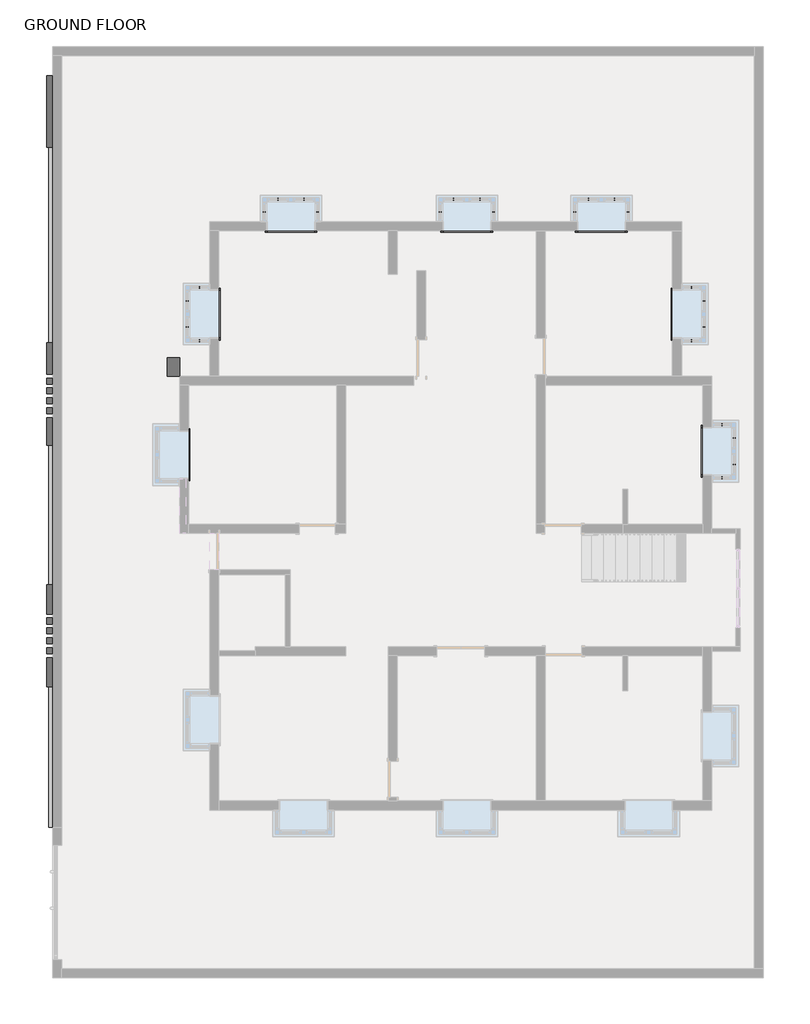
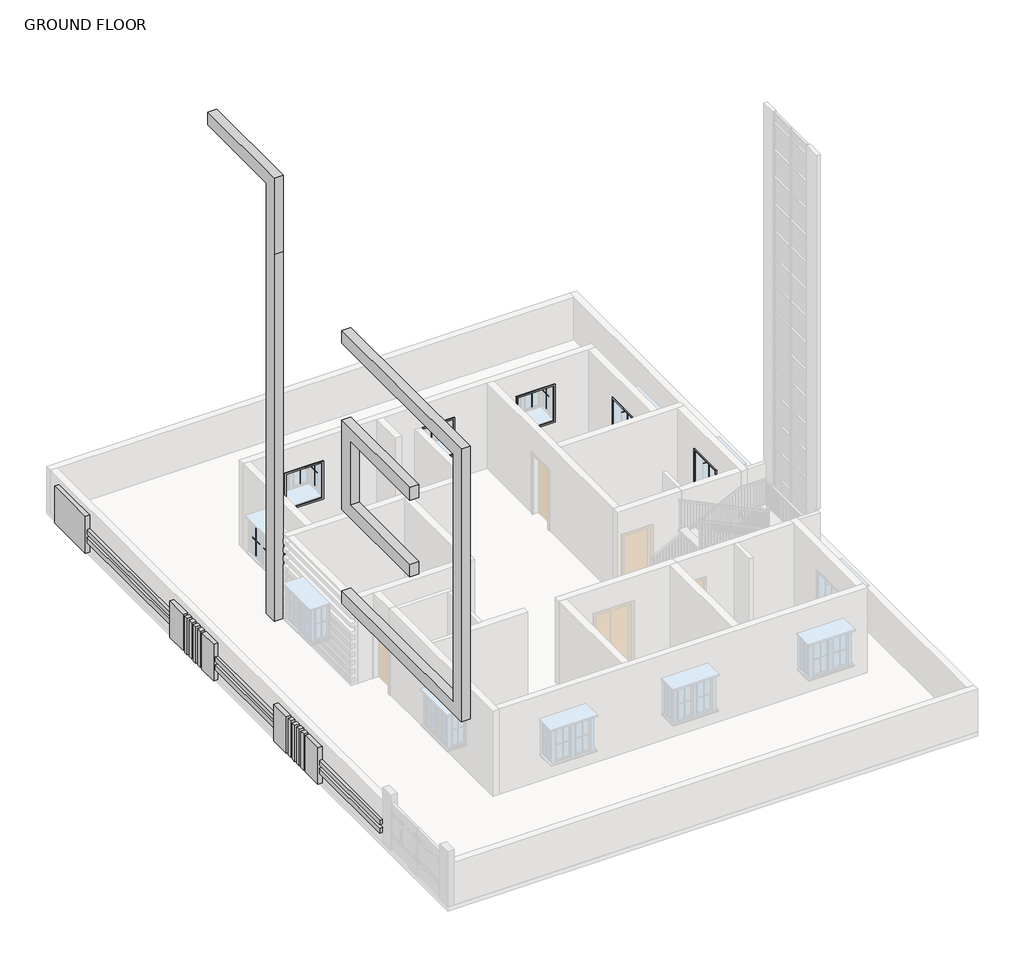
# One storey, part 5 of 5: 32 proxies.
"""IFC4 building model written with IfcOpenShell, lengths in millimetres."""

from ifc_helpers import new_model, si_unit, origin, place, context, project, spatial, transform, mapped, element, save
from components import generic_models_2_generic_models_2_d91b4525, muntin_pattern_2x2_muntin_pattern_2x2_4aee108e, muntin_pattern_2x2_muntin_pattern_2x2_f03ab90d, muntin_pattern_2x2_muntin_pattern_2x2_eb08c668, trim_window_interior_flat_picture_frame_ace0ae79

model = new_model("IFC4")

# Units and contexts
model_context = context("Model", 3, world=origin())
ifc_project = project(units=[si_unit("LENGTHUNIT", "METRE", prefix="MILLI")], contexts=[model_context])

# Site, building, storey
site = spatial("IfcSite", under=ifc_project)
building = spatial("IfcBuilding", under=site)
storey = spatial("IfcBuildingStorey", under=building, Name="GROUND FLOOR", Elevation=0.0)

# Proxies
placement = place(None, origin())
generic_models_2_generic_models_2_shape = generic_models_2_generic_models_2_d91b4525(model_context)
element("IfcBuildingElementProxy", 1, Name="Generic Models 2 : Generic Models 2", ObjectType="Generic Models 2 : Generic Models 2", at=placement, inside=storey, context=model_context, shape_type="MappedRepresentation", body=[
    mapped(generic_models_2_generic_models_2_shape, transform((0.0, 0.0, 0.0), x_axis=(1.0, 0.0, 0.0), y_axis=(0.0, 1.0, 0.0), z_axis=(0.0, 0.0, 1.0))),
])
muntin_pattern_2x2_muntin_pattern_2x2_shape = muntin_pattern_2x2_muntin_pattern_2x2_4aee108e(model_context)
element("IfcBuildingElementProxy", 2, Name="Muntin Pattern_2x2 : Muntin Pattern_2x2", ObjectType="Muntin Pattern_2x2 : Muntin Pattern_2x2", at=placement, inside=storey, context=model_context, shape_type="MappedRepresentation", body=[
    mapped(muntin_pattern_2x2_muntin_pattern_2x2_shape, transform((6209.1834916, 6075.433346, 1035.05), x_axis=(0.0, -1.0, 0.0), y_axis=(1.0, 0.0, 0.0), z_axis=(0.0, 0.0, 1.0))),
])
element("IfcBuildingElementProxy", 3, Name="Muntin Pattern_2x2 : Muntin Pattern_2x2", ObjectType="Muntin Pattern_2x2 : Muntin Pattern_2x2", at=placement, inside=storey, context=model_context, shape_type="MappedRepresentation", body=[
    mapped(muntin_pattern_2x2_muntin_pattern_2x2_shape, transform((-6814.6665084, 5415.033346, 1035.05), x_axis=(0.0, 1.0, 0.0), y_axis=(-1.0, 0.0, 0.0), z_axis=(0.0, 0.0, 1.0))),
])
element("IfcBuildingElementProxy", 4, Name="Muntin Pattern_2x2 : Muntin Pattern_2x2", ObjectType="Muntin Pattern_2x2 : Muntin Pattern_2x2", at=placement, inside=storey, context=model_context, shape_type="MappedRepresentation", body=[
    mapped(muntin_pattern_2x2_muntin_pattern_2x2_shape, transform((-99.5415084, 8637.658346, 1035.05), x_axis=(1.0, 0.0, 0.0), y_axis=(0.0, 1.0, 0.0), z_axis=(0.0, 0.0, 1.0))),
])
element("IfcBuildingElementProxy", 5, Name="Muntin Pattern_2x2 : Muntin Pattern_2x2", ObjectType="Muntin Pattern_2x2 : Muntin Pattern_2x2", at=placement, inside=storey, context=model_context, shape_type="MappedRepresentation", body=[
    mapped(muntin_pattern_2x2_muntin_pattern_2x2_shape, transform((3291.3584916, 8637.658346, 1035.05), x_axis=(1.0, 0.0, 0.0), y_axis=(0.0, 1.0, 0.0), z_axis=(0.0, 0.0, 1.0))),
])
element("IfcBuildingElementProxy", 6, Name="Muntin Pattern_2x2 : Muntin Pattern_2x2", ObjectType="Muntin Pattern_2x2 : Muntin Pattern_2x2", at=placement, inside=storey, context=model_context, shape_type="MappedRepresentation", body=[
    mapped(muntin_pattern_2x2_muntin_pattern_2x2_shape, transform((-4531.8415084, 8637.658346, 1035.05), x_axis=(1.0, 0.0, 0.0), y_axis=(0.0, 1.0, 0.0), z_axis=(0.0, 0.0, 1.0))),
])
element("IfcBuildingElementProxy", 7, Name="Muntin Pattern_2x2 : Muntin Pattern_2x2", ObjectType="Muntin Pattern_2x2 : Muntin Pattern_2x2", at=placement, inside=storey, context=model_context, shape_type="MappedRepresentation", body=[
    mapped(muntin_pattern_2x2_muntin_pattern_2x2_shape, transform((6971.1834916, 2621.033346, 1035.05), x_axis=(0.0, -1.0, 0.0), y_axis=(1.0, 0.0, 0.0), z_axis=(0.0, 0.0, 1.0))),
])
muntin_pattern_2x2_muntin_pattern_2x2_2_shape = muntin_pattern_2x2_muntin_pattern_2x2_f03ab90d(model_context)
element("IfcBuildingElementProxy", 8, Name="Muntin Pattern_2x2 : Muntin Pattern_2x2", ObjectType="Muntin Pattern_2x2 : Muntin Pattern_2x2", at=placement, inside=storey, context=model_context, shape_type="MappedRepresentation", body=[
    mapped(muntin_pattern_2x2_muntin_pattern_2x2_2_shape, transform((5894.8584916, 6415.158346, 1035.05), x_axis=(-1.0, 0.0, 0.0), y_axis=(0.0, -1.0, 0.0), z_axis=(0.0, 0.0, 1.0))),
])
element("IfcBuildingElementProxy", 9, Name="Muntin Pattern_2x2 : Muntin Pattern_2x2", ObjectType="Muntin Pattern_2x2 : Muntin Pattern_2x2", at=placement, inside=storey, context=model_context, shape_type="MappedRepresentation", body=[
    mapped(muntin_pattern_2x2_muntin_pattern_2x2_2_shape, transform((5894.8584916, 5075.308346, 1035.05), x_axis=(1.0, 0.0, 0.0), y_axis=(0.0, 1.0, 0.0), z_axis=(0.0, 0.0, 1.0))),
])
element("IfcBuildingElementProxy", 10, Name="Muntin Pattern_2x2 : Muntin Pattern_2x2", ObjectType="Muntin Pattern_2x2 : Muntin Pattern_2x2", at=placement, inside=storey, context=model_context, shape_type="MappedRepresentation", body=[
    mapped(muntin_pattern_2x2_muntin_pattern_2x2_2_shape, transform((-6500.3415084, 5075.308346, 1035.05), x_axis=(1.0, 0.0, 0.0), y_axis=(0.0, 1.0, 0.0), z_axis=(0.0, 0.0, 1.0))),
])
element("IfcBuildingElementProxy", 11, Name="Muntin Pattern_2x2 : Muntin Pattern_2x2", ObjectType="Muntin Pattern_2x2 : Muntin Pattern_2x2", at=placement, inside=storey, context=model_context, shape_type="MappedRepresentation", body=[
    mapped(muntin_pattern_2x2_muntin_pattern_2x2_2_shape, transform((-6500.3415084, 6415.158346, 1035.05), x_axis=(-1.0, 0.0, 0.0), y_axis=(0.0, -1.0, 0.0), z_axis=(0.0, 0.0, 1.0))),
])
element("IfcBuildingElementProxy", 12, Name="Muntin Pattern_2x2 : Muntin Pattern_2x2", ObjectType="Muntin Pattern_2x2 : Muntin Pattern_2x2", at=placement, inside=storey, context=model_context, shape_type="MappedRepresentation", body=[
    mapped(muntin_pattern_2x2_muntin_pattern_2x2_2_shape, transform((-439.2665084, 8323.333346, 1035.05), x_axis=(0.0, -1.0, 0.0), y_axis=(1.0, 0.0, 0.0), z_axis=(0.0, 0.0, 1.0))),
])
element("IfcBuildingElementProxy", 13, Name="Muntin Pattern_2x2 : Muntin Pattern_2x2", ObjectType="Muntin Pattern_2x2 : Muntin Pattern_2x2", at=placement, inside=storey, context=model_context, shape_type="MappedRepresentation", body=[
    mapped(muntin_pattern_2x2_muntin_pattern_2x2_2_shape, transform((900.5834916, 8323.333346, 1035.05), x_axis=(0.0, 1.0, 0.0), y_axis=(-1.0, 0.0, 0.0), z_axis=(0.0, 0.0, 1.0))),
])
element("IfcBuildingElementProxy", 14, Name="Muntin Pattern_2x2 : Muntin Pattern_2x2", ObjectType="Muntin Pattern_2x2 : Muntin Pattern_2x2", at=placement, inside=storey, context=model_context, shape_type="MappedRepresentation", body=[
    mapped(muntin_pattern_2x2_muntin_pattern_2x2_2_shape, transform((2951.6334916, 8323.333346, 1035.05), x_axis=(0.0, -1.0, 0.0), y_axis=(1.0, 0.0, 0.0), z_axis=(0.0, 0.0, 1.0))),
])
element("IfcBuildingElementProxy", 15, Name="Muntin Pattern_2x2 : Muntin Pattern_2x2", ObjectType="Muntin Pattern_2x2 : Muntin Pattern_2x2", at=placement, inside=storey, context=model_context, shape_type="MappedRepresentation", body=[
    mapped(muntin_pattern_2x2_muntin_pattern_2x2_2_shape, transform((4291.4834916, 8323.333346, 1035.05), x_axis=(0.0, 1.0, 0.0), y_axis=(-1.0, 0.0, 0.0), z_axis=(0.0, 0.0, 1.0))),
])
element("IfcBuildingElementProxy", 16, Name="Muntin Pattern_2x2 : Muntin Pattern_2x2", ObjectType="Muntin Pattern_2x2 : Muntin Pattern_2x2", at=placement, inside=storey, context=model_context, shape_type="MappedRepresentation", body=[
    mapped(muntin_pattern_2x2_muntin_pattern_2x2_2_shape, transform((-4871.5665084, 8323.333346, 1035.05), x_axis=(0.0, -1.0, 0.0), y_axis=(1.0, 0.0, 0.0), z_axis=(0.0, 0.0, 1.0))),
])
element("IfcBuildingElementProxy", 17, Name="Muntin Pattern_2x2 : Muntin Pattern_2x2", ObjectType="Muntin Pattern_2x2 : Muntin Pattern_2x2", at=placement, inside=storey, context=model_context, shape_type="MappedRepresentation", body=[
    mapped(muntin_pattern_2x2_muntin_pattern_2x2_2_shape, transform((-3531.7165084, 8323.333346, 1035.05), x_axis=(0.0, 1.0, 0.0), y_axis=(-1.0, 0.0, 0.0), z_axis=(0.0, 0.0, 1.0))),
])
element("IfcBuildingElementProxy", 18, Name="Muntin Pattern_2x2 : Muntin Pattern_2x2", ObjectType="Muntin Pattern_2x2 : Muntin Pattern_2x2", at=placement, inside=storey, context=model_context, shape_type="MappedRepresentation", body=[
    mapped(muntin_pattern_2x2_muntin_pattern_2x2_2_shape, transform((6656.8584916, 2960.758346, 1035.05), x_axis=(-1.0, 0.0, 0.0), y_axis=(0.0, -1.0, 0.0), z_axis=(0.0, 0.0, 1.0))),
])
element("IfcBuildingElementProxy", 19, Name="Muntin Pattern_2x2 : Muntin Pattern_2x2", ObjectType="Muntin Pattern_2x2 : Muntin Pattern_2x2", at=placement, inside=storey, context=model_context, shape_type="MappedRepresentation", body=[
    mapped(muntin_pattern_2x2_muntin_pattern_2x2_2_shape, transform((6656.8584916, 1620.908346, 1035.05), x_axis=(1.0, 0.0, 0.0), y_axis=(0.0, 1.0, 0.0), z_axis=(0.0, 0.0, 1.0))),
])
muntin_pattern_2x2_muntin_pattern_2x2_3_shape = muntin_pattern_2x2_muntin_pattern_2x2_eb08c668(model_context)
element("IfcBuildingElementProxy", 20, Name="Muntin Pattern_2x2 : Muntin Pattern_2x2", ObjectType="Muntin Pattern_2x2 : Muntin Pattern_2x2", at=placement, inside=storey, context=model_context, shape_type="MappedRepresentation", body=[
    mapped(muntin_pattern_2x2_muntin_pattern_2x2_3_shape, transform((6209.1834916, 5415.033346, 1035.05), x_axis=(0.0, 1.0, 0.0), y_axis=(-1.0, 0.0, 0.0), z_axis=(0.0, 0.0, 1.0))),
])
element("IfcBuildingElementProxy", 21, Name="Muntin Pattern_2x2 : Muntin Pattern_2x2", ObjectType="Muntin Pattern_2x2 : Muntin Pattern_2x2", at=placement, inside=storey, context=model_context, shape_type="MappedRepresentation", body=[
    mapped(muntin_pattern_2x2_muntin_pattern_2x2_3_shape, transform((-6814.6665084, 6075.433346, 1035.05), x_axis=(0.0, -1.0, 0.0), y_axis=(1.0, 0.0, 0.0), z_axis=(0.0, 0.0, 1.0))),
])
element("IfcBuildingElementProxy", 22, Name="Muntin Pattern_2x2 : Muntin Pattern_2x2", ObjectType="Muntin Pattern_2x2 : Muntin Pattern_2x2", at=placement, inside=storey, context=model_context, shape_type="MappedRepresentation", body=[
    mapped(muntin_pattern_2x2_muntin_pattern_2x2_3_shape, transform((560.8584916, 8637.658346, 1035.05), x_axis=(-1.0, 0.0, 0.0), y_axis=(0.0, -1.0, 0.0), z_axis=(0.0, 0.0, 1.0))),
])
element("IfcBuildingElementProxy", 23, Name="Muntin Pattern_2x2 : Muntin Pattern_2x2", ObjectType="Muntin Pattern_2x2 : Muntin Pattern_2x2", at=placement, inside=storey, context=model_context, shape_type="MappedRepresentation", body=[
    mapped(muntin_pattern_2x2_muntin_pattern_2x2_3_shape, transform((3951.7584916, 8637.658346, 1035.05), x_axis=(-1.0, 0.0, 0.0), y_axis=(0.0, -1.0, 0.0), z_axis=(0.0, 0.0, 1.0))),
])
element("IfcBuildingElementProxy", 24, Name="Muntin Pattern_2x2 : Muntin Pattern_2x2", ObjectType="Muntin Pattern_2x2 : Muntin Pattern_2x2", at=placement, inside=storey, context=model_context, shape_type="MappedRepresentation", body=[
    mapped(muntin_pattern_2x2_muntin_pattern_2x2_3_shape, transform((-3871.4415084, 8637.658346, 1035.05), x_axis=(-1.0, 0.0, 0.0), y_axis=(0.0, -1.0, 0.0), z_axis=(0.0, 0.0, 1.0))),
])
element("IfcBuildingElementProxy", 25, Name="Muntin Pattern_2x2 : Muntin Pattern_2x2", ObjectType="Muntin Pattern_2x2 : Muntin Pattern_2x2", at=placement, inside=storey, context=model_context, shape_type="MappedRepresentation", body=[
    mapped(muntin_pattern_2x2_muntin_pattern_2x2_3_shape, transform((6971.1834916, 1960.633346, 1035.05), x_axis=(0.0, 1.0, 0.0), y_axis=(-1.0, 0.0, 0.0), z_axis=(0.0, 0.0, 1.0))),
])
trim_window_interior_flat_picture_frame_shape = trim_window_interior_flat_picture_frame_ace0ae79(model_context)
element("IfcBuildingElementProxy", 26, Name="Trim-Window-Interior-Flat : Picture Frame", ObjectType="Trim-Window-Interior-Flat : Picture Frame", at=placement, inside=storey, context=model_context, shape_type="MappedRepresentation", body=[
    mapped(trim_window_interior_flat_picture_frame_shape, transform((5412.2584916, 5745.233346, 2184.4), x_axis=(0.0, -1.0, 0.0), y_axis=(0.0, 0.0, 1.0), z_axis=(-1.0, 0.0, 0.0))),
])
element("IfcBuildingElementProxy", 27, Name="Trim-Window-Interior-Flat : Picture Frame", ObjectType="Trim-Window-Interior-Flat : Picture Frame", at=placement, inside=storey, context=model_context, shape_type="MappedRepresentation", body=[
    mapped(trim_window_interior_flat_picture_frame_shape, transform((-6017.7415084, 5745.233346, 2184.4), x_axis=(0.0, 1.0, 0.0), y_axis=(0.0, 0.0, 1.0), z_axis=(1.0, 0.0, 0.0))),
])
element("IfcBuildingElementProxy", 28, Name="Trim-Window-Interior-Flat : Picture Frame", ObjectType="Trim-Window-Interior-Flat : Picture Frame", at=placement, inside=storey, context=model_context, shape_type="MappedRepresentation", body=[
    mapped(trim_window_interior_flat_picture_frame_shape, transform((230.6584916, 7840.733346, 2184.4), x_axis=(1.0, 0.0, 0.0), y_axis=(0.0, 0.0, 1.0), z_axis=(0.0, -1.0, 0.0))),
])
element("IfcBuildingElementProxy", 29, Name="Trim-Window-Interior-Flat : Picture Frame", ObjectType="Trim-Window-Interior-Flat : Picture Frame", at=placement, inside=storey, context=model_context, shape_type="MappedRepresentation", body=[
    mapped(trim_window_interior_flat_picture_frame_shape, transform((3621.5584916, 7840.733346, 2184.4), x_axis=(1.0, 0.0, 0.0), y_axis=(0.0, 0.0, 1.0), z_axis=(0.0, -1.0, 0.0))),
])
element("IfcBuildingElementProxy", 30, Name="Trim-Window-Interior-Flat : Picture Frame", ObjectType="Trim-Window-Interior-Flat : Picture Frame", at=placement, inside=storey, context=model_context, shape_type="MappedRepresentation", body=[
    mapped(trim_window_interior_flat_picture_frame_shape, transform((-4201.6415084, 7840.733346, 2184.4), x_axis=(1.0, 0.0, 0.0), y_axis=(0.0, 0.0, 1.0), z_axis=(0.0, -1.0, 0.0))),
])
element("IfcBuildingElementProxy", 31, Name="Trim-Window-Interior-Flat : Picture Frame", ObjectType="Trim-Window-Interior-Flat : Picture Frame", at=placement, inside=storey, context=model_context, shape_type="MappedRepresentation", body=[
    mapped(trim_window_interior_flat_picture_frame_shape, transform((-6779.7415084, 2201.933346, 2184.4), x_axis=(0.0, 1.0, 0.0), y_axis=(0.0, 0.0, 1.0), z_axis=(1.0, 0.0, 0.0))),
])
element("IfcBuildingElementProxy", 32, Name="Trim-Window-Interior-Flat : Picture Frame", ObjectType="Trim-Window-Interior-Flat : Picture Frame", at=placement, inside=storey, context=model_context, shape_type="MappedRepresentation", body=[
    mapped(trim_window_interior_flat_picture_frame_shape, transform((6174.2584916, 2290.833346, 2184.4), x_axis=(0.0, -1.0, 0.0), y_axis=(0.0, 0.0, 1.0), z_axis=(-1.0, 0.0, 0.0))),
])

save(model, "model.ifc")

# Revit data of these elements
# Type "Muntin Pattern_2x2 : Muntin Pattern_2x2"
#   Width [instance default] = 4' - 0"
#   Thickness = 0' - 0 1/2"
#   Height [instance default] = 4' - 0"
#   Distance = 0' - 0 3/4"
#   Interior Material [instance default] = none
#   Exterior Material [instance default] = none
#   Default Elevation = 0
# Type "Trim-Window-Interior-Flat : Picture Frame"
#   Trim Thickness_Picture Frame = 0' - 1 1/4"
#   Trim Width = 0' - 2 1/4"
#   Trim Thickness_with Sill = 0' - 0 3/4"
#   Sill Thickness = 0' - 1 1/4"
#   Opening Width [instance default] = 2' - 0"
#   Opening Height [instance default] = 3' - 0"
#   Default Elevation = 4' - 0"
#   Sill = no
#   Picture Frame = yes
#   Trim Material [instance default] = none
# Element 1 (IfcBuildingElementProxy, "Generic Models 2 : Generic Models 2")
#   Phase Created = New Construction
#   Materials on its faces: "Wood Planks", "GATE"
# Elements 2, 3, 4, 5, 6, 7, 20, 21, 22, 23, 24, 25 (IfcBuildingElementProxy, "Muntin Pattern_2x2 : Muntin Pattern_2x2")
#   Width = 1' - 4 1/2"
#   Height = 3' - 6 1/2"
#   Interior Material = Wood - Stained
#   Exterior Material = Clad - White
#   Phase Created = New Construction
#   Materials on its faces: "Clad - White", "Wood - Stained"
# Elements 8, 9, 10, 11, 12, 13, 14, 15, 16, 17, 18, 19 (IfcBuildingElementProxy, "Muntin Pattern_2x2 : Muntin Pattern_2x2")
#   Width = 1' - 2 1/2"
#   Height = 3' - 6 1/2"
#   Interior Material = Wood - Stained
#   Exterior Material = Clad - White
#   Phase Created = New Construction
#   Materials on its faces: "Clad - White", "Wood - Stained"
# Elements 26, 27, 28, 29, 30, 31, 32 (IfcBuildingElementProxy, "Trim-Window-Interior-Flat : Picture Frame")
#   Opening Width = 4' - 0"
#   Opening Height = 4' - 2"
#   Trim Material = Wood - Stained
#   Phase Created = New Construction
#   Materials on its faces: "Wood - Stained"
# Materials
#   "Wood Planks": class "Wood", colour RGB 193 160 115, transparency 0, Description = "Physical material.", Cost = 0
#   "GATE": class "Generic", colour RGB 120 120 120, transparency 0, Cost = 0
#   "Clad - White": class "Wood", colour RGB 242 242 238, transparency 0, Cost = 0
#   "Wood - Stained": class "Wood", colour RGB 224 178 126, transparency 0, Cost = 0
